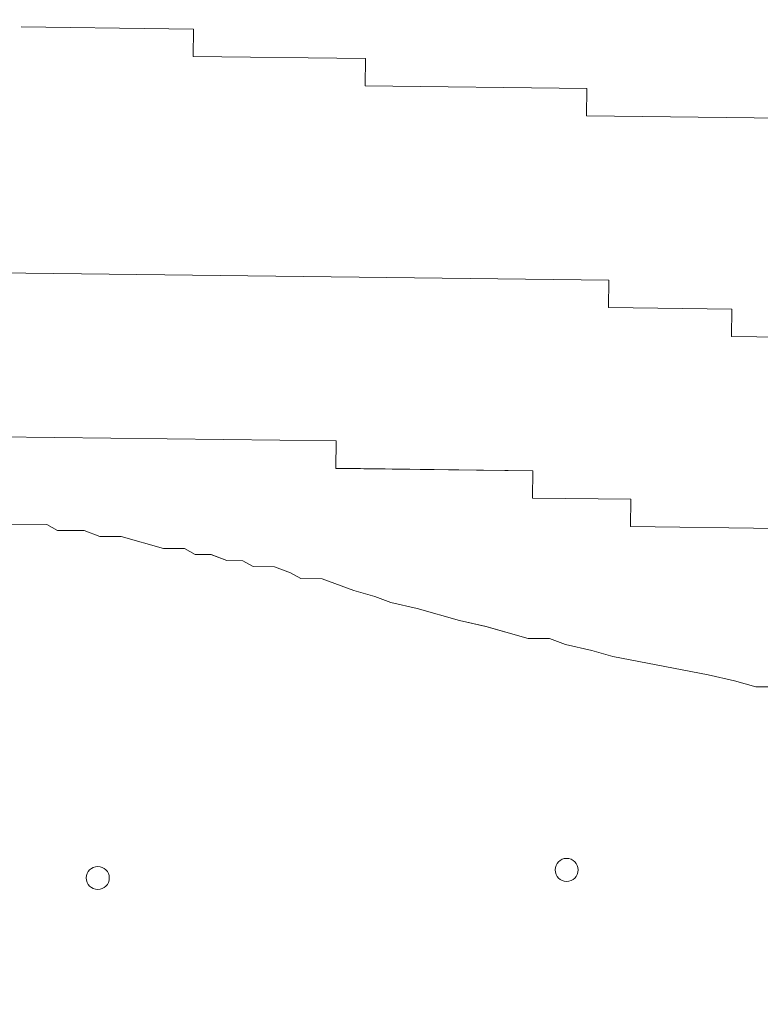
# Model space of a CAD drawing. Units: inches. Extents: x -466983 to 1020, y 324 to 318697.
# Tile 76 of 97: x 652.495 to 656.235, y 939.297 to 944.271. Entities that reach past the tile are written whole.
import ezdxf

# ---------------------------------------------------------------- set-up
doc = ezdxf.new("R2010")
doc.units = ezdxf.units.IN
doc.header["$MEASUREMENT"] = 0
doc.layers.add('A-FLOR-PATT', color=252, linetype='Continuous', lineweight=13)
doc.layers.add('A-FURN', color=8, linetype='Continuous', lineweight=18)

# ---------------------------------------------------------------- blocks, each defined once
blk = doc.blocks.new('L Shaped Sofa')
at = {"ltscale": 2}
for p, q in [((2395.89, 747.0093), (2396.0851, 747.0084)), ((2396.0851, 747.0084), (2396.28, 746.9532)), ((2396.28, 746.9532), (2396.5236, 746.8979)), ((2396.5236, 746.8979), (2397.4009, 746.7311)), ((2397.4009, 746.7311), (2397.5958, 746.676)), ((2397.5958, 746.676), (2397.8394, 746.6206)), ((2397.8394, 746.6206), (2397.9855, 746.5657)), ((2397.9855, 746.5657), (2398.1807, 746.5648)), ((2398.1807, 746.5648), (2398.5704, 746.4545)), ((2398.5704, 746.4545), (2398.814, 746.3992)), ((2398.814, 746.3992), (2399.2037, 746.2889)), ((2399.2037, 746.2889), (2399.4473, 746.2335)), ((2399.4473, 746.2335), (2399.5934, 746.1786)), ((2399.5934, 746.1786), (2399.7883, 746.1235)), ((2399.7883, 746.1235), (2400.0804, 746.0137)), ((2400.0804, 746.0137), (2400.2755, 746.0128)), ((2400.2755, 746.0128), (2400.3728, 745.9581)), ((2400.3728, 745.9581), (2400.5188, 745.9032)), ((2400.5188, 745.9032), (2400.714, 745.9023)), ((2400.714, 745.9023), (2400.8113, 745.8476)), ((2400.8113, 745.8476), (2400.9577, 745.8469)), ((2400.9577, 745.8469), (2401.1037, 745.792)), ((2401.1037, 745.792), (2401.2501, 745.7913)), ((2401.2501, 745.7913), (2401.3474, 745.7367)), ((2401.3474, 745.7367), (2401.5426, 745.7357)), ((2401.5426, 745.7357), (2401.9322, 745.6255)), ((2401.9322, 745.6255), (2402.1274, 745.6246)), ((2402.1274, 745.6246), (2402.2735, 745.5697)), ((2402.2735, 745.5697), (2402.5175, 745.5685)), ((2402.5175, 745.5685), (2402.6147, 745.5138)), ((2395.8772, 745.5504), (2397.2382, 745.5337)), ((2397.2382, 745.5337), (2397.2352, 745.2818)), ((2402.6147, 745.5138), (2403.0051, 745.512)), ((2397.2352, 745.2818), (2398.1425, 745.2707)), ((2398.1425, 745.2707), (2398.1394, 745.0188)), ((2398.1394, 745.0188), (2399.9541, 744.9967)), ((2399.9541, 744.9967), (2399.951, 744.7447)), ((2399.951, 744.7447), (2403.5804, 744.7004)), ((2395.1752, 743.7953), (2396.3094, 743.7814)), ((2396.3094, 743.7814), (2396.3063, 743.5295)), ((2396.3063, 743.5295), (2397.4405, 743.5157)), ((2397.4405, 743.5157), (2397.4374, 743.2638)), ((2397.4374, 743.2638), (2403.562, 743.1889)), ((2392.4285, 741.8133), (2397.6457, 741.7495)), ((2397.6457, 741.7495), (2397.6427, 741.4976)), ((2397.6427, 741.4976), (2399.6842, 741.4727)), ((2399.6842, 741.4727), (2399.6811, 741.2207)), ((2399.6811, 741.2207), (2401.269, 741.2013)), ((2401.269, 741.2013), (2401.2659, 740.9494)), ((2401.2659, 740.9494), (2401.7196, 740.9439)), ((2401.4927, 740.9467), (2402.8538, 740.93)), ((2401.7196, 740.9439), (2401.4927, 740.9467))]:
    blk.add_line(p, q, dxfattribs=at)
for centre, start, end in [((2402.1467, 748.7712), 90, 270), ((2402.1467, 748.7712), 270, 90), ((2397.8273, 748.697), 90, 270), ((2397.8273, 748.697), 270, 90)]:
    blk.add_arc(centre, 0.1062, start, end, dxfattribs=at)

msp = doc.modelspace()

# ---------------------------------------------------------------- hatches: boundary and pattern name
at = {"layer": 'A-FLOR-PATT', "transparency": 33554572}
h = msp.add_hatch(dxfattribs=at)
h.set_pattern_fill('ANSI37', color=256, scale=30)
h.set_pattern_definition([(45, (-1212.4137, -290.035), (-2.6516504, 2.6516504), []), (135, (-1212.4137, -290.035), (-2.6516504, -2.6516504), [])])
h.paths.add_polyline_path([(901.8057, 1075.9377), (900.6144, 1075.9377), (900.6144, 1065.3856), (899.391, 1065.3856), (898.0911, 1065.3856), (892.8356, 1058.7098, -0.258377), (892.1875, 1058.3509), (879.9848, 1058.3509, -0.20177), (879.4382, 1058.5808), (874.0812, 1065.3856), (872.7813, 1065.3856), (871.5579, 1065.3856), (871.5579, 1075.9377), (813.8057, 1075.9377), (813.8057, 1044.7922), (832.3947, 1044.7922, -0.394795), (848.6602, 1028.5356), (848.6602, 1009.9377), (901.8057, 1009.9377), (901.8057, 1015.9377), (901.3057, 1015.9377), (871.3057, 1015.9377), (871.3057, 1017.2502), (871.3344, 1017.2502, -0.401453), (901.3057, 1045.9377), (901.8057, 1045.9377)])
edge = h.paths.add_edge_path(flags=16)
edge.add_line((847.7731, 1068.9486), (847.7731, 1073.7088))
edge.add_arc((849.2269, 1073.7088), 1.4538, 90, 180, ccw=False)
edge.add_line((849.2269, 1075.1627), (864.4921, 1075.1627))
edge.add_arc((864.4921, 1073.7088), 1.4538, 0, 90, ccw=False)
edge.add_line((865.9459, 1073.7088), (865.9459, 1069.0035))
edge.add_arc((832.6447, 1068.9761), 33.3012, -20.61234, 0.04725, ccw=False)
edge.add_ellipse((856.8595, 1058.48), major_axis=(0, 10.2131), ratio=0.6859192, start_angle=100.00884, end_angle=259.99116, ccw=False)
edge.add_arc((881.0742, 1068.9761), 33.3012, 180.04725, 200.61234, ccw=False)
h.paths.add_polyline_path([(853.1456, 1066.4815), (853.1456, 1066.4534), (853.1463, 1066.4534, 0.433107), (852.9166, 1066.6849), (852.9166, 1066.4534), (853.1456, 1066.4534), (853.1456, 1066.4815), (853.088, 1066.6122, 0.697939), (852.6995, 1066.4534), (852.7003, 1066.4534), (852.7003, 1066.4815), (852.9166, 1067.0012), (852.9166, 1066.6849, -0.396254)], flags=0)
h.paths.add_polyline_path([(861.0187, 1066.4815), (861.0187, 1066.4534), (861.0194, 1066.4534, 0.416404), (860.8024, 1066.6849), (860.8024, 1066.4534), (861.0187, 1066.4534), (861.0187, 1066.4815), (860.9672, 1066.6053, 0.713344), (860.5726, 1066.4534), (860.5734, 1066.4534), (860.5734, 1066.4815), (860.8024, 1067.0012), (860.8024, 1066.6849, -0.379973)], flags=0)
edge = h.paths.add_edge_path(flags=0)
edge.add_spline(control_points=[(861.1298, 1065.7855), (861.4661, 1065.2478), (861.6134, 1065.0161), (861.9833, 1064.3736), (862.1924, 1063.9443), (862.5614, 1063.0391), (862.7212, 1062.5633), (862.9865, 1061.5781), (863.092, 1061.0689), (863.2452, 1060.031), (863.293, 1059.5025), (863.3295, 1058.4409), (863.3181, 1057.9078), (863.2366, 1056.8518), (863.1664, 1056.3289), (862.9695, 1055.308), (862.8427, 1054.8099), (862.5365, 1053.8522), (862.3571, 1053.3927), (861.9514, 1052.5249), (861.7251, 1052.1166), (861.233, 1051.3622), (860.9672, 1051.0162), (860.4048, 1050.3949), (860.1082, 1050.1197), (859.4937, 1049.6461), (859.1758, 1049.4476), (858.5276, 1049.1299), (858.1973, 1049.0107), (857.5315, 1048.8518), (857.1959, 1048.8121), (856.5249, 1048.812), (856.1894, 1048.8515), (855.5236, 1049.0101), (855.1933, 1049.1291), (854.545, 1049.4465), (854.2271, 1049.6449), (853.6124, 1050.1183), (853.3158, 1050.3933), (852.7533, 1051.0143), (852.4874, 1051.3602), (851.9952, 1052.1144), (851.7688, 1052.5225), (851.3629, 1053.3902), (851.1834, 1053.8496), (850.877, 1054.8071), (850.7501, 1055.3051), (850.553, 1056.326), (850.4827, 1056.8488), (850.401, 1057.9048), (850.3895, 1058.4379), (850.4257, 1059.4995), (850.4734, 1060.0281), (850.6265, 1061.066), (850.7318, 1061.5753), (850.9969, 1062.5605), (851.1567, 1063.0365), (851.5254, 1063.9418), (851.7345, 1064.3712), (852.1056, 1065.0164), (852.2544, 1065.2503), (852.6082, 1065.7335)], knot_values=[3.915332, 3.915332, 3.915332, 3.915332, 4.013468, 4.013468, 4.175532, 4.175532, 4.337596, 4.337596, 4.49966, 4.49966, 4.661724, 4.661724, 4.823788, 4.823788, 4.985852, 4.985852, 5.147916, 5.147916, 5.30998, 5.30998, 5.472044, 5.472044, 5.634109, 5.634109, 5.796173, 5.796173, 5.958237, 5.958237, 6.120301, 6.120301, 6.282365, 6.282365, 6.444429, 6.444429, 6.606493, 6.606493, 6.768557, 6.768557, 6.930621, 6.930621, 7.092685, 7.092685, 7.254749, 7.254749, 7.416813, 7.416813, 7.578878, 7.578878, 7.740942, 7.740942, 7.903006, 7.903006, 8.06507, 8.06507, 8.227134, 8.227134, 8.389198, 8.389198, 8.551262, 8.551262, 8.65037, 8.65037, 8.65037, 8.65037], degree=3, periodic=0)
edge.add_line((852.6421, 1065.7855), (861.1298, 1065.7855))
edge = h.paths.add_edge_path(flags=0)
edge.add_ellipse((856.8496, 1057.7432), major_axis=(0, 7.7921), ratio=0.687861, start_angle=0, end_angle=360)
h.paths.add_polyline_path([(848.8634, 1069.3891), (848.8634, 1073.9605, -0.414214), (849.9538, 1075.0508), (863.7652, 1075.0508, -0.414214), (864.8555, 1073.9605), (864.8555, 1069.3891, -0.388936), (864.5237, 1069.027, -0.043561), (849.1953, 1069.027, -0.388936)], flags=0)
h.paths.add_polyline_path([(853.1006, 1068.1122, -1), (852.6775, 1068.1122, -1)], flags=0)
edge = h.paths.add_edge_path(flags=0)
edge.add_ellipse((856.8595, 1057.3378), major_axis=(0, 2.207), ratio=0.657164, start_angle=0, end_angle=360)
h.paths.add_polyline_path([(861.0415, 1068.1122, -1), (860.6184, 1068.1122, -1)], flags=0)
edge = h.paths.add_edge_path()
edge.add_line((573.9537, 1057.3412), (573.9537, 1075.9377))
edge.add_line((573.9537, 1075.9377), (558.7308, 1075.9377))
edge.add_line((558.7308, 1075.9377), (558.7308, 1065.3856))
edge.add_line((558.7308, 1065.3856), (557.5074, 1065.3856))
edge.add_line((557.5074, 1065.3856), (556.2075, 1065.3856))
edge.add_line((556.2075, 1065.3856), (550.952, 1058.7098))
edge.add_arc((550.3039, 1059.1155), 0.7646, 270, 327.9483, ccw=False)
edge.add_line((550.3039, 1058.3509), (538.1012, 1058.3509))
edge.add_arc((538.1012, 1059.1155), 0.7646, 224.3704, 270, ccw=False)
edge.add_line((537.5546, 1058.5808), (532.1976, 1065.3856))
edge.add_line((532.1976, 1065.3856), (530.8977, 1065.3856))
edge.add_line((530.8977, 1065.3856), (529.6743, 1065.3856))
edge.add_line((529.6743, 1065.3856), (529.6743, 1075.9377))
edge.add_line((529.6743, 1075.9377), (520.8057, 1075.9377))
edge.add_line((520.8057, 1075.9377), (520.8057, 1045.9377))
edge.add_line((520.8057, 1045.9377), (521.3057, 1045.9377))
edge.add_arc((521.3057, 1015.9377), 30, 2.50749, 90, ccw=False)
edge.add_line((551.277, 1017.2502), (551.3057, 1017.2502))
edge.add_line((551.3057, 1017.2502), (551.3057, 1015.9377))
edge.add_line((551.3057, 1015.9377), (520.8057, 1015.9377))
edge.add_line((520.8057, 1015.9377), (520.8057, 1009.9377))
edge.add_line((520.8057, 1009.9377), (559.1913, 1010.4022))
edge.add_arc((559.1913, 1011.856), 1.4538, 180, 270, ccw=False)
edge.add_line((557.7375, 1011.856), (557.7375, 1016.5613))
edge.add_arc((591.0386, 1016.5888), 33.3012, 159.38766, 180.04725, ccw=False)
edge.add_ellipse((566.8239, 1027.0848), major_axis=(0, 10.2131), ratio=0.6859192, start_angle=280.00884, end_angle=439.99116, ccw=False)
edge.add_arc((542.6091, 1016.5888), 33.3012, 0.04725, 20.61234, ccw=False)
edge.add_line((575.9103, 1016.6162), (575.9103, 1011.856))
edge.add_arc((574.4565, 1011.856), 1.4538, -90, 0, ccw=False)
edge.add_line((574.4565, 1010.4022), (608.8057, 1009.9377))
edge.add_line((608.8057, 1009.9377), (608.8057, 1041.0857))
edge.add_line((608.8057, 1041.0857), (590.2179, 1041.0857))
edge.add_arc((590.775, 1057.9074), 16.8309, 181.92775, 268.10321, ccw=False)
edge = h.paths.add_edge_path()
edge.add_ellipse((494.2443, 583.6204), major_axis=(0, 10.2131), ratio=0.6859192, start_angle=280.00884, end_angle=439.99116, ccw=False)
edge.add_arc((470.0296, 573.1243), 33.3012, 0.04725, 20.61234, ccw=False)
edge.add_line((503.3307, 573.1518), (503.3307, 568.3916))
edge.add_arc((501.8769, 568.3916), 1.4538, -90, 0, ccw=False)
edge.add_line((501.8769, 566.9377), (539.8057, 566.9377))
edge.add_line((539.8057, 566.9377), (539.8057, 572.9377))
edge.add_line((539.8057, 572.9377), (539.3057, 572.9377))
edge.add_line((539.3057, 572.9377), (509.3057, 572.9377))
edge.add_line((509.3057, 572.9377), (509.3057, 574.2502))
edge.add_line((509.3057, 574.2502), (509.3344, 574.2502))
edge.add_arc((539.3057, 572.9377), 30, 90, 177.49251, ccw=False)
edge.add_line((539.3057, 602.9377), (539.8057, 602.9377))
edge.add_line((539.8057, 602.9377), (539.8057, 626.9377))
edge.add_line((539.8057, 626.9377), (531.7718, 626.9377))
edge.add_line((531.7718, 626.9377), (531.7718, 616.3856))
edge.add_line((531.7718, 616.3856), (530.5484, 616.3856))
edge.add_line((530.5484, 616.3856), (529.2485, 616.3856))
edge.add_line((529.2485, 616.3856), (523.7105, 609.3509))
edge.add_line((523.7105, 609.3509), (510.7766, 609.3509))
edge.add_line((510.7766, 609.3509), (505.2386, 616.3856))
edge.add_line((505.2386, 616.3856), (503.9387, 616.3856))
edge.add_line((503.9387, 616.3856), (502.7153, 616.3856))
edge.add_line((502.7153, 616.3856), (502.7153, 626.9377))
edge.add_line((502.7153, 626.9377), (481.6983, 626.9377))
edge.add_line((481.6983, 626.9377), (481.6983, 610.995))
edge.add_arc((467.2703, 611.4728), 14.4359, 271.92775, 358.10321, ccw=False)
edge.add_line((467.7559, 597.0451), (451.8057, 597.0451))
edge.add_line((451.8057, 597.0451), (451.8057, 584.4035))
edge.add_line((451.8057, 584.4035), (451.8057, 566.9377))
edge.add_line((451.8057, 566.9377), (486.6117, 566.9377))
edge.add_arc((486.6117, 568.3916), 1.4538, 180, 270, ccw=False)
edge.add_line((485.1579, 568.3916), (485.1579, 573.0969))
edge.add_arc((518.4591, 573.1243), 33.3012, 159.38766, 180.04725, ccw=False)
h.paths.add_polyline_path([(836.2609, 1020.7328), (879.8898, 1020.7328), (879.8898, 1039.3902), (836.2609, 1039.3902)], flags=25)
h.paths.add_polyline_path([(549.9851, 1036.7492), (593.614, 1036.7492), (593.614, 1055.4065), (549.9851, 1055.4065)], flags=24)
h.paths.add_polyline_path([(475.123, 595.5959), (518.752, 595.5959), (518.752, 614.2532), (475.123, 614.2532)], flags=24)
h = msp.add_hatch(dxfattribs=at)
h.set_pattern_fill('ANSI37', color=256, scale=20)
h.set_pattern_definition([(45, (-1212.4137, -290.035), (-1.767767, 1.767767), []), (135, (-1212.4137, -290.035), (-1.767767, -1.767767), [])])
h.paths.add_polyline_path([(809.8057, 870.9377), (809.8057, 888.1519), (806.9985, 888.1519), (802.6624, 888.1519), (789.3832, 888.1519), (786.2846, 888.1519, -0.414214), (785.4991, 888.9374), (785.4991, 900.1959), (785.4991, 908.4696, -0.414214), (786.8082, 909.7787, -0.414214), (785.4991, 911.0878), (785.4991, 929.1015, -0.414214), (786.8082, 930.4106, -0.414214), (785.4991, 931.7197), (785.4991, 931.9039, -0.414214), (784.19, 930.5948), (766.7223, 930.5948, -0.412359), (765.4132, 931.8956, -0.413741), (764.1145, 930.5782), (744.5781, 930.422, -0.416556), (743.7864, 931.2075), (743.7864, 933.5153), (742.2154, 933.5153), (742.2154, 952.024, -0.001344), (743.7864, 952.1998), (743.7864, 953.9377), (678.5915, 953.9377), (678.5915, 951.1305), (678.5915, 946.7945), (678.5915, 933.5153), (678.5915, 930.4166, -0.414214), (677.806, 929.6312), (666.5475, 929.6312), (658.2738, 929.6312, -0.414214), (656.9647, 930.9403, -0.414214), (655.6556, 929.6312), (637.6419, 929.6312, -0.414214), (636.3328, 930.9403, -0.414214), (635.0237, 929.6312), (634.8395, 929.6312, -0.414214), (636.1486, 928.322), (636.1486, 910.8544, -0.412359), (634.8478, 909.5452, -0.413741), (636.1653, 908.2466), (636.3214, 888.7102, -0.416556), (635.5359, 887.9184), (633.2281, 887.9184), (633.2281, 886.3475), (614.7194, 886.3475, -0.001344), (614.5436, 887.9184), (612.8057, 887.9184), (612.8057, 834.9377), (612.8057, 752.9377), (612.8057, 748.9377), (612.8057, 697.9377), (654.8057, 697.9377), (654.8057, 701.9377), (715.8057, 701.9377), (715.8057, 737.4353), (774.2918, 737.4353), (774.2918, 795.9377), (809.8057, 795.9377)])
h.paths.add_polyline_path([(679.2761, 849.5757, 0.102523), (682.1475, 849.2608, -0.080461), (694.5428, 849.7725, -0.283899), (694.4822, 849.0082, 0.136605), (694.4068, 848.8103, -0.030441), (694.5428, 846.8929), (694.5428, 842.6198), (694.5428, 838.3466, -0.028219), (694.4246, 836.5684), (694.425, 836.5684, 0.196187), (694.4456, 836.2708, -0.302897), (694.5428, 835.467, -0.080461), (682.1475, 835.9787, 0.102523), (679.2761, 835.6638, -0.58611), (678.6457, 836.0169), (678.6457, 849.2227, -0.58611)], flags=16)
h.paths.add_polyline_path([(679.5173, 848.6515, 0.699597), (679.476, 848.6342, 1.20716), (679.1935, 848.7422, 0.010621)], flags=0)
h.paths.add_polyline_path([(679.4923, 836.5608, -0.013798), (679.9178, 836.6594, -0.071703), (682.8533, 837.1434, -0.165743), (682.1665, 839.1006), (682.1665, 842.6094), (682.1665, 846.0603, -0.240616), (683.4733, 848.6767, -0.068263), (693.9295, 849.0082), (693.7875, 848.7083), (693.7875, 849.0228, 0.067332), (683.4733, 848.6767, 0.240616), (682.1665, 846.0603), (682.1665, 842.6094), (682.1665, 839.1006, 0.23459), (683.461, 836.5513, 0.068093), (693.7875, 836.1955), (693.7875, 836.5104), (693.9296, 836.2102, -0.077215), (682.2421, 836.7815, 0.086627), (679.5283, 836.5701, -0.628402), (679.5029, 836.5735), (679.5029, 836.6071, 0.910458)], flags=0)
h.paths.add_polyline_path([(679.476, 848.6364), (679.2069, 848.647), (679.2069, 836.5718, 0.913566), (679.3645, 836.5861), (679.476, 836.5824)], flags=0)
h.paths.add_polyline_path([(679.2761, 829.8604, 0.102523), (682.1475, 829.5455, -0.080461), (694.5428, 830.0572, -0.283899), (694.4822, 829.2929, 0.136605), (694.4068, 829.095, -0.030441), (694.5428, 827.1776), (694.5428, 822.9045), (694.5428, 818.6314, -0.028219), (694.4246, 816.8531), (694.425, 816.8532, 0.196187), (694.4456, 816.5555, -0.302897), (694.5428, 815.7517, -0.080461), (682.1475, 816.2635, 0.102523), (679.2761, 815.9485, -0.58611), (678.6457, 816.3016), (678.6457, 829.5074, -0.58611)], flags=16)
h.paths.add_polyline_path([(679.5173, 828.9362, 0.699597), (679.476, 828.9189, 1.20716), (679.1935, 829.0269, 0.010621)], flags=0)
h.paths.add_polyline_path([(679.4923, 816.8456, -0.013798), (679.9178, 816.9441, -0.071703), (682.8533, 817.4281, -0.165743), (682.1665, 819.3853), (682.1665, 822.8941), (682.1665, 826.345, -0.240616), (683.4733, 828.9614, -0.068263), (693.9295, 829.2929), (693.7875, 828.9931), (693.7875, 829.3076, 0.067332), (683.4733, 828.9614, 0.240616), (682.1665, 826.345), (682.1665, 822.8941), (682.1665, 819.3853, 0.23459), (683.461, 816.836, 0.068093), (693.7875, 816.4802), (693.7875, 816.7952), (693.9296, 816.4949, -0.077215), (682.2421, 817.0662, 0.086627), (679.5283, 816.8549, -0.628402), (679.5029, 816.8582), (679.5029, 816.8918, 0.910458)], flags=0)
h.paths.add_polyline_path([(679.476, 828.9211), (679.2069, 828.9317), (679.2069, 816.8565, 0.913566), (679.3645, 816.8708), (679.476, 816.8671)], flags=0)
h.paths.add_polyline_path([(679.2761, 810.1451, 0.102523), (682.1475, 809.8302, -0.080461), (694.5428, 810.342, -0.3023), (694.4466, 809.5394, 0.10023), (694.4058, 809.3878, -0.03057), (694.5428, 807.4623), (694.5428, 803.1892), (694.5428, 798.9161, -0.03057), (694.4058, 796.9906, 0.10023), (694.4466, 796.839, -0.3023), (694.5428, 796.0365, -0.080461), (682.1475, 796.5482, 0.102523), (679.2761, 796.2333, -0.58611), (678.6457, 796.5863), (678.6457, 809.7921, -0.58611)], flags=16)
h.paths.add_polyline_path([(679.5173, 809.2417, 0.699597), (679.476, 809.2244, 1.20716), (679.1935, 809.3324, 0.010621)], flags=0)
h.paths.add_polyline_path([(679.4923, 797.151, -0.013798), (679.9178, 797.2496, -0.071703), (682.8533, 797.7336, -0.165743), (682.1665, 799.6908), (682.1665, 803.1996), (682.1665, 806.6505, -0.239349), (683.461, 809.2577, -0.072465), (694.4468, 809.5405, 0.197932), (694.425, 809.2405), (693.7875, 809.2985), (693.7875, 809.6135, 0.068093), (683.461, 809.2577, 0.239349), (682.1665, 806.6505), (682.1665, 803.1996), (682.1665, 799.6908, 0.235854), (683.4733, 797.1323, 0.067332), (693.7875, 796.7861), (693.7875, 797.1006), (694.425, 797.1586, 0.197932), (694.4468, 796.8586, -0.080419), (682.1557, 797.3795, 0.083867), (679.5283, 797.1603, -0.628402), (679.5029, 797.1637), (679.5029, 797.1973, 0.910458)], flags=0)
h.paths.add_polyline_path([(679.2069, 809.2372), (679.2069, 797.162, 0.913566), (679.3645, 797.1763), (679.476, 797.1726), (679.476, 809.2266)], flags=0)
h.paths.add_polyline_path([(695.3643, 853.2989), (728.2231, 853.2989), (728.2231, 771.1519), (695.3643, 771.1519)], flags=16)
h.paths.add_polyline_path([(696.0215, 852.6417), (727.5659, 852.6417), (727.5659, 771.809), (696.0215, 771.809)], flags=0)
h.paths.add_polyline_path([(679.2761, 788.7869, 0.102523), (682.1475, 788.472, -0.080461), (694.5428, 788.9837, -0.3023), (694.4466, 788.1812, 0.10023), (694.4058, 788.0296, -0.03057), (694.5428, 786.1041), (694.5428, 781.831), (694.5428, 777.5578, -0.03057), (694.4058, 775.6323, 0.10023), (694.4466, 775.4808, -0.3023), (694.5428, 774.6782, -0.080461), (682.1475, 775.19, 0.102523), (679.2761, 774.875, -0.58611), (678.6457, 775.2281), (678.6457, 788.4339, -0.58611)], flags=16)
h.paths.add_polyline_path([(679.5173, 787.8834, 0.699597), (679.476, 787.8662, 1.20716), (679.1935, 787.9742, 0.010621)], flags=0)
h.paths.add_polyline_path([(679.4923, 775.7928, -0.013798), (679.9178, 775.8914, -0.071703), (682.8533, 776.3753, -0.165743), (682.1665, 778.3325), (682.1665, 781.8414), (682.1665, 785.2922, -0.239349), (683.461, 787.8995, -0.072465), (694.4468, 788.1823, 0.197932), (694.425, 787.8823), (693.7875, 787.9403), (693.7875, 788.2553, 0.068093), (683.461, 787.8995, 0.239349), (682.1665, 785.2922), (682.1665, 781.8414), (682.1665, 778.3325, 0.235854), (683.4733, 775.7741, 0.067332), (693.7875, 775.4279), (693.7875, 775.7424), (694.425, 775.8004, 0.197932), (694.4468, 775.5004, -0.080419), (682.1557, 776.0212, 0.083867), (679.5283, 775.8021, -0.628402), (679.5029, 775.8054), (679.5029, 775.8391, 0.910458)], flags=0)
h.paths.add_polyline_path([(679.2069, 787.8789), (679.2069, 775.8038, 0.913566), (679.3645, 775.818), (679.476, 775.8144), (679.476, 787.8684)], flags=0)
h.paths.add_polyline_path([(704.641, 854.1204, -0.080461), (705.1527, 866.5157, 0.102523), (704.8378, 869.3871, -0.58611), (705.1908, 870.0174), (718.3966, 870.0174, -0.58611), (718.7496, 869.3871, 0.102523), (718.4347, 866.5157, -0.080461), (718.9465, 854.1204, -0.3023), (718.1439, 854.2166, 0.10023), (717.9924, 854.2574, -0.03057), (716.0668, 854.1204), (711.7937, 854.1204), (707.5206, 854.1204, -0.03057), (705.5951, 854.2574, 0.10023), (705.4435, 854.2166, -0.3023)], flags=16)
h.paths.add_polyline_path([(717.8462, 869.1459, 0.699597), (717.8289, 869.1872, 1.20716), (717.9369, 869.4697, 0.010621)], flags=0)
h.paths.add_polyline_path([(705.4631, 854.2164, -0.080419), (705.984, 866.5074, 0.083867), (705.7648, 869.1349, -0.628402), (705.7682, 869.1603), (705.8018, 869.1603, 0.910458), (705.7555, 869.1709, -0.013798), (705.8541, 868.7454, -0.071703), (706.3381, 865.8099, -0.165743), (708.2953, 866.4967), (711.8041, 866.4967), (715.255, 866.4967, -0.239349), (717.8622, 865.2022, -0.072465), (718.145, 854.2164, 0.197932), (717.845, 854.2382), (717.903, 854.8757), (718.218, 854.8757, 0.068093), (717.8622, 865.2022, 0.239349), (715.255, 866.4967), (711.8041, 866.4967), (708.2953, 866.4967, 0.235854), (705.7368, 865.1898, 0.067332), (705.3906, 854.8757), (705.7051, 854.8757), (705.7631, 854.2382, 0.197932)], flags=16)
h.paths.add_polyline_path([(705.7665, 869.4563, 0.913566), (705.7808, 869.2987), (705.7771, 869.1872), (717.8311, 869.1872), (717.8417, 869.4563)], flags=0)
h.paths.add_polyline_path([(729.0446, 842.6198), (729.0446, 846.8929, -0.03057), (729.1817, 848.8184, 0.10023), (729.1408, 848.9699, -0.3023), (729.0446, 849.7725, -0.080461), (741.4399, 849.2608, 0.102523), (744.3113, 849.5757, -0.58611), (744.9417, 849.2227), (744.9417, 836.0169, -0.58611), (744.3113, 835.6638, 0.102523), (741.4399, 835.9787, -0.080461), (729.0446, 835.467, -0.3023), (729.1408, 836.2696, 0.10023), (729.1817, 836.4211, -0.03057), (729.0446, 838.3466)], flags=16)
h.paths.add_polyline_path([(744.1115, 836.5846, 1.20716), (744.3939, 836.4766, 0.010621), (744.0701, 836.5673, 0.699597)], flags=0)
h.paths.add_polyline_path([(729.1407, 836.2684, 0.197932), (729.1624, 836.5684), (729.7999, 836.5104), (729.7999, 836.1955, 0.068093), (740.1264, 836.5513, 0.239349), (741.4209, 839.1585), (741.4209, 842.6094), (741.4209, 846.1182, 0.235854), (740.1141, 848.6767, 0.067332), (729.7999, 849.0228), (729.7999, 848.7083), (729.1624, 848.6503, 0.197932), (729.1407, 848.9504, -0.080419), (741.4317, 848.4295, 0.083867), (744.0591, 848.6486, -0.628402), (744.0845, 848.6453), (744.0845, 848.6117, 0.910458), (744.0951, 848.6579, -0.013798), (743.6696, 848.5594, -0.071703), (740.7341, 848.0754, -0.165743), (741.4209, 846.1182), (741.4209, 842.6094), (741.4209, 839.1585, -0.239349), (740.1264, 836.5513, -0.072465)], flags=0)
h.paths.add_polyline_path([(729.0446, 830.0572, -0.080461), (741.4399, 829.5455, 0.102523), (744.3113, 829.8604, -0.58611), (744.9417, 829.5074), (744.9417, 816.3016, -0.58611), (744.3113, 815.9485, 0.102523), (741.4399, 816.2635, -0.080461), (729.0446, 815.7517, -0.3023), (729.1408, 816.5543, 0.10023), (729.1817, 816.7058, -0.03057), (729.0446, 818.6314), (729.0446, 822.9045), (729.0446, 827.1776, -0.03057), (729.1817, 829.1031, 0.10023), (729.1408, 829.2547, -0.3023)], flags=16)
h.paths.add_polyline_path([(744.1115, 816.8693, 1.20716), (744.3939, 816.7613, 0.010621), (744.0701, 816.852, 0.699597)], flags=0)
h.paths.add_polyline_path([(729.1407, 829.2351, -0.080419), (741.4317, 828.7142, 0.083867), (744.0591, 828.9334, -0.628402), (744.0845, 828.93), (744.0845, 828.8964, 0.910458), (744.0951, 828.9427, -0.013798), (743.6696, 828.8441, -0.071703), (740.7341, 828.3601, -0.165743), (741.4209, 826.4029), (741.4209, 822.8941), (741.4209, 819.4432, -0.239349), (740.1264, 816.836, -0.072465), (729.1407, 816.5531, 0.197932), (729.1624, 816.8532), (729.7999, 816.7952), (729.7999, 816.4802, 0.068093), (740.1264, 816.836, 0.239349), (741.4209, 819.4432), (741.4209, 822.8941), (741.4209, 826.4029, 0.235854), (740.1141, 828.9614, 0.067332), (729.7999, 829.3076), (729.7999, 828.9931), (729.1624, 828.9351, 0.197932)], flags=16)
h.paths.add_polyline_path([(729.0446, 810.342, -0.080461), (741.4399, 809.8302, 0.102523), (744.3113, 810.1451, -0.58611), (744.9417, 809.7921), (744.9417, 796.5863, -0.58611), (744.3113, 796.2333, 0.102523), (741.4399, 796.5482, -0.080461), (729.0446, 796.0365, -0.283899), (729.1052, 796.8007, 0.136605), (729.1806, 796.9987, -0.030441), (729.0446, 798.9161), (729.0446, 803.1892), (729.0446, 807.4623, -0.028219), (729.1628, 809.2406), (729.1624, 809.2405, 0.196187), (729.1418, 809.5382, -0.302897)], flags=16)
h.paths.add_polyline_path([(744.1115, 797.1748, 1.20716), (744.3939, 797.0668, 0.010621), (744.0701, 797.1575, 0.699597)], flags=0)
h.paths.add_polyline_path([(741.3453, 809.0275, 0.086627), (744.0591, 809.2388, -0.628402), (744.0845, 809.2355), (744.0845, 809.2019, 0.910458), (744.0951, 809.2481, -0.013798), (743.6696, 809.1496, -0.071703), (740.7341, 808.6656, -0.165743), (741.4209, 806.7084), (741.4209, 803.1996), (741.4209, 799.7487, -0.240616), (740.1141, 797.1323, -0.068263), (729.658, 796.8008), (729.7999, 797.1006), (729.7999, 796.7861, 0.067332), (740.1141, 797.1323, 0.240616), (741.4209, 799.7487), (741.4209, 803.1996), (741.4209, 806.7084, 0.23459), (740.1264, 809.2577, 0.068093), (729.7999, 809.6135), (729.7999, 809.2985), (729.6578, 809.5988, -0.077215)], flags=0)
h.paths.add_polyline_path([(704.641, 770.3304, -0.283899), (705.4053, 770.2697, 0.136605), (705.6032, 770.1944, -0.030441), (707.5206, 770.3304), (711.7937, 770.3304), (716.0668, 770.3304, -0.028219), (717.8451, 770.2122), (717.845, 770.2126, 0.196187), (718.1427, 770.2331, -0.302897), (718.9465, 770.3304, -0.080461), (718.4347, 757.9351, 0.102523), (718.7496, 755.0637, -0.58611), (718.3966, 754.4333), (705.1908, 754.4333, -0.58611), (704.8378, 755.0637, 0.102523), (705.1527, 757.9351, -0.080461)], flags=16)
h.paths.add_polyline_path([(705.762, 755.3048, 0.699597), (705.7793, 755.2635, 1.20716), (705.6713, 754.9811, 0.010621)], flags=0)
h.paths.add_polyline_path([(705.4053, 769.717), (705.7051, 769.5751), (705.3906, 769.5751, 0.067332), (705.7368, 759.2609, 0.240616), (708.3532, 757.954), (711.8041, 757.954), (715.3129, 757.954, 0.23459), (717.8622, 759.2485, 0.068093), (718.218, 769.5751), (717.903, 769.5751), (718.2033, 769.7172, -0.077215), (717.632, 758.0297, 0.086627), (717.8433, 755.3159, -0.628402), (717.84, 755.2904), (717.8064, 755.2904, 0.910458), (717.8526, 755.2799, -0.013798), (717.7541, 755.7053, -0.071703), (717.2701, 758.6409, -0.165743), (715.3129, 757.954), (711.8041, 757.954), (708.3532, 757.954, -0.240616), (705.7368, 759.2609, -0.068263)], flags=0)
h.paths.add_polyline_path([(729.0446, 788.9837, -0.080461), (741.4399, 788.472, 0.102523), (744.3113, 788.7869, -0.58611), (744.9417, 788.4339), (744.9417, 775.2281, -0.58611), (744.3113, 774.875, 0.102523), (741.4399, 775.19, -0.080461), (729.0446, 774.6782, -0.283899), (729.1052, 775.4425, 0.136605), (729.1806, 775.6405, -0.030441), (729.0446, 777.5578), (729.0446, 781.831), (729.0446, 786.1041, -0.028219), (729.1628, 787.8823), (729.1624, 787.8823, 0.196187), (729.1418, 788.1799, -0.302897)], flags=16)
h.paths.add_polyline_path([(744.1115, 775.8165, 1.20716), (744.3939, 775.7086, 0.010621), (744.0701, 775.7993, 0.699597)], flags=0)
h.paths.add_polyline_path([(741.3453, 787.6692, 0.086627), (744.0591, 787.8806, -0.628402), (744.0845, 787.8773), (744.0845, 787.8437, 0.910458), (744.0951, 787.8899, -0.013798), (743.6696, 787.7913, -0.071703), (740.7341, 787.3074, -0.165743), (741.4209, 785.3502), (741.4209, 781.8414), (741.4209, 778.3905, -0.240616), (740.1141, 775.7741, -0.068263), (729.658, 775.4425), (729.7999, 775.7424), (729.7999, 775.4279, 0.067332), (740.1141, 775.7741, 0.240616), (741.4209, 778.3905), (741.4209, 781.8414), (741.4209, 785.3502, 0.23459), (740.1264, 787.8995, 0.068093), (729.7999, 788.2553), (729.7999, 787.9403), (729.6578, 788.2405, -0.077215)], flags=0)
h.paths.add_polyline_path([(744.1115, 848.6364), (744.1115, 836.5824), (744.3805, 836.5718), (744.3805, 848.647, 0.913566), (744.2229, 848.6327)], flags=0)
h.paths.add_polyline_path([(744.2229, 828.9174), (744.1115, 828.9211), (744.1115, 816.8671), (744.3805, 816.8565), (744.3805, 828.9317, 0.913566)], flags=0)
h.paths.add_polyline_path([(717.8311, 755.2635), (705.7771, 755.2635), (705.7665, 754.9945), (717.8417, 754.9945, 0.913566), (717.8274, 755.1521)], flags=0)
h.paths.add_polyline_path([(744.2229, 809.2229), (744.1115, 809.2266), (744.1115, 797.1726), (744.3805, 797.162), (744.3805, 809.2372, 0.913566)], flags=0)
h.paths.add_polyline_path([(744.1115, 787.8684), (744.1115, 775.8144), (744.3805, 775.8038), (744.3805, 787.8789, 0.913566), (744.2229, 787.8647)], flags=0)
h.paths.add_polyline_path([(678.8774, 877.1228), (737.6127, 877.1228), (737.6127, 899.5116), (678.8774, 899.5116)], flags=24)

# ---------------------------------------------------------------- linework, layer by layer
at = {"layer": 'A-FURN', "ltscale": 2}
for p, q in [((653.2476, 944.2249), (652.5014, 944.234)), ((653.2476, 944.2249), (652.5014, 944.234)), ((653.2476, 944.2249), (652.5014, 944.234)), ((653.2476, 944.2249), (652.5014, 944.234)), ((653.2476, 944.2249), (652.5014, 944.234)), ((653.2476, 944.2249), (652.5014, 944.234)), ((653.1232, 944.2264), (653.2476, 944.2249)), ((653.3719, 944.2233), (653.1232, 944.2264)), ((653.1232, 944.2264), (653.2476, 944.2249)), ((653.3719, 944.2233), (653.1232, 944.2264)), ((653.1232, 944.2264), (653.2476, 944.2249)), ((653.3719, 944.2233), (653.1232, 944.2264)), ((653.1232, 944.2264), (653.2476, 944.2249)), ((653.3719, 944.2233), (653.1232, 944.2264)), ((653.1232, 944.2264), (653.2476, 944.2249)), ((653.3719, 944.2233), (653.1232, 944.2264)), ((653.1232, 944.2264), (653.2476, 944.2249)), ((653.3719, 944.2233), (653.1232, 944.2264)), ((653.3702, 944.0852), (653.3719, 944.2233)), ((653.3702, 944.0852), (653.3719, 944.2233)), ((653.3702, 944.0852), (653.3719, 944.2233)), ((653.3702, 944.0852), (653.3719, 944.2233)), ((653.3702, 944.0852), (653.3719, 944.2233)), ((653.3702, 944.0852), (653.3719, 944.2233)), ((654.2407, 944.0746), (653.3702, 944.0852)), ((654.2407, 944.0746), (653.3702, 944.0852)), ((654.2407, 944.0746), (653.3702, 944.0852)), ((654.2407, 944.0746), (653.3702, 944.0852)), ((654.2407, 944.0746), (653.3702, 944.0852)), ((654.2407, 944.0746), (653.3702, 944.0852)), ((654.239, 943.9365), (654.2407, 944.0746)), ((654.239, 943.9365), (654.2407, 944.0746)), ((654.239, 943.9365), (654.2407, 944.0746)), ((654.239, 943.9365), (654.2407, 944.0746)), ((654.239, 943.9365), (654.2407, 944.0746)), ((654.239, 943.9365), (654.2407, 944.0746)), ((655.3582, 943.9228), (654.239, 943.9365)), ((655.3582, 943.9228), (654.239, 943.9365)), ((655.3582, 943.9228), (654.239, 943.9365)), ((655.3582, 943.9228), (654.239, 943.9365)), ((655.3582, 943.9228), (654.239, 943.9365)), ((655.3582, 943.9228), (654.239, 943.9365)), ((655.3565, 943.7847), (655.3582, 943.9228)), ((655.3565, 943.7847), (655.3582, 943.9228)), ((655.3565, 943.7847), (655.3582, 943.9228)), ((655.3565, 943.7847), (655.3582, 943.9228)), ((655.3565, 943.7847), (655.3582, 943.9228)), ((655.3565, 943.7847), (655.3582, 943.9228)), ((658.2167, 943.7498), (655.3565, 943.7847)), ((658.2167, 943.7498), (655.3565, 943.7847)), ((658.2167, 943.7498), (655.3565, 943.7847)), ((658.2167, 943.7498), (655.3565, 943.7847)), ((658.2167, 943.7498), (655.3565, 943.7847)), ((658.2167, 943.7498), (655.3565, 943.7847)), ((655.4708, 942.9546), (652.1132, 942.9956)), ((655.4708, 942.9546), (652.1132, 942.9956)), ((655.4708, 942.9546), (652.1132, 942.9956)), ((655.4708, 942.9546), (652.1132, 942.9956)), ((655.4708, 942.9546), (652.1132, 942.9956)), ((655.4708, 942.9546), (652.1132, 942.9956)), ((655.4691, 942.8165), (655.4708, 942.9546)), ((655.4691, 942.8165), (655.4708, 942.9546)), ((655.4691, 942.8165), (655.4708, 942.9546)), ((655.4691, 942.8165), (655.4708, 942.9546)), ((655.4691, 942.8165), (655.4708, 942.9546)), ((655.4691, 942.8165), (655.4708, 942.9546)), ((656.0909, 942.8089), (655.4691, 942.8165)), ((656.0909, 942.8089), (655.4691, 942.8165)), ((656.0909, 942.8089), (655.4691, 942.8165)), ((656.0909, 942.8089), (655.4691, 942.8165)), ((656.0909, 942.8089), (655.4691, 942.8165)), ((656.0909, 942.8089), (655.4691, 942.8165)), ((656.0892, 942.6708), (656.0909, 942.8089)), ((656.0892, 942.6708), (656.0909, 942.8089)), ((656.0892, 942.6708), (656.0909, 942.8089)), ((656.0892, 942.6708), (656.0909, 942.8089)), ((656.0892, 942.6708), (656.0909, 942.8089)), ((656.0892, 942.6708), (656.0909, 942.8089)), ((656.711, 942.6632), (656.0892, 942.6708)), ((656.711, 942.6632), (656.0892, 942.6708)), ((656.711, 942.6632), (656.0892, 942.6708)), ((656.711, 942.6632), (656.0892, 942.6708)), ((656.711, 942.6632), (656.0892, 942.6708)), ((656.711, 942.6632), (656.0892, 942.6708)), ((654.0927, 942.1427), (652.1031, 942.167)), ((654.0927, 942.1427), (652.1031, 942.167)), ((654.0927, 942.1427), (652.1031, 942.167)), ((654.0927, 942.1427), (652.1031, 942.167)), ((654.0927, 942.1427), (652.1031, 942.167)), ((654.0927, 942.1427), (652.1031, 942.167)), ((654.0911, 942.0046), (654.0927, 942.1427)), ((654.0911, 942.0046), (654.0927, 942.1427)), ((654.0911, 942.0046), (654.0927, 942.1427)), ((654.0911, 942.0046), (654.0927, 942.1427)), ((654.0911, 942.0046), (654.0927, 942.1427)), ((654.0911, 942.0046), (654.0927, 942.1427)), ((655.0859, 941.9924), (654.0911, 942.0046)), ((655.0859, 941.9924), (654.0911, 942.0046)), ((655.0859, 941.9924), (654.0911, 942.0046)), ((655.0859, 941.9924), (654.0911, 942.0046)), ((655.0859, 941.9924), (654.0911, 942.0046)), ((655.0859, 941.9924), (654.0911, 942.0046)), ((655.0842, 941.8543), (655.0859, 941.9924)), ((655.0842, 941.8543), (655.0859, 941.9924)), ((655.0842, 941.8543), (655.0859, 941.9924)), ((655.0842, 941.8543), (655.0859, 941.9924)), ((655.0842, 941.8543), (655.0859, 941.9924)), ((655.0842, 941.8543), (655.0859, 941.9924)), ((655.5816, 941.8483), (655.0842, 941.8543)), ((655.5816, 941.8483), (655.0842, 941.8543)), ((655.5816, 941.8483), (655.0842, 941.8543)), ((655.5816, 941.8483), (655.0842, 941.8543)), ((655.5816, 941.8483), (655.0842, 941.8543)), ((655.5816, 941.8483), (655.0842, 941.8543)), ((655.5799, 941.7102), (655.5816, 941.8483)), ((655.5799, 941.7102), (655.5816, 941.8483)), ((655.5799, 941.7102), (655.5816, 941.8483)), ((655.5799, 941.7102), (655.5816, 941.8483)), ((655.5799, 941.7102), (655.5816, 941.8483)), ((655.5799, 941.7102), (655.5816, 941.8483)), ((652.6325, 941.7211), (652.4185, 941.7221)), ((652.6325, 941.7211), (652.4185, 941.7221)), ((652.6325, 941.7211), (652.4185, 941.7221)), ((652.6325, 941.7211), (652.4185, 941.7221)), ((652.6325, 941.7211), (652.4185, 941.7221)), ((652.6325, 941.7211), (652.4185, 941.7221)), ((652.6858, 941.6911), (652.6325, 941.7211)), ((652.6858, 941.6911), (652.6325, 941.7211)), ((652.6858, 941.6911), (652.6325, 941.7211)), ((652.6858, 941.6911), (652.6325, 941.7211)), ((652.6858, 941.6911), (652.6325, 941.7211)), ((652.6858, 941.6911), (652.6325, 941.7211)), ((656.3261, 941.701), (655.5799, 941.7102)), ((656.3261, 941.701), (655.5799, 941.7102)), ((656.3261, 941.701), (655.5799, 941.7102)), ((656.3261, 941.701), (655.5799, 941.7102)), ((656.3261, 941.701), (655.5799, 941.7102)), ((656.3261, 941.701), (655.5799, 941.7102)), ((652.8195, 941.6905), (652.6858, 941.6911)), ((652.8195, 941.6905), (652.6858, 941.6911)), ((652.8195, 941.6905), (652.6858, 941.6911)), ((652.8195, 941.6905), (652.6858, 941.6911)), ((652.8195, 941.6905), (652.6858, 941.6911)), ((652.8195, 941.6905), (652.6858, 941.6911)), ((652.8996, 941.6604), (652.8195, 941.6905)), ((652.8996, 941.6604), (652.8195, 941.6905)), ((652.8996, 941.6604), (652.8195, 941.6905)), ((652.8996, 941.6604), (652.8195, 941.6905)), ((652.8996, 941.6604), (652.8195, 941.6905)), ((652.8996, 941.6604), (652.8195, 941.6905)), ((653.0066, 941.6599), (652.8996, 941.6604)), ((653.0066, 941.6599), (652.8996, 941.6604)), ((653.0066, 941.6599), (652.8996, 941.6604)), ((653.0066, 941.6599), (652.8996, 941.6604)), ((653.0066, 941.6599), (652.8996, 941.6604)), ((653.0066, 941.6599), (652.8996, 941.6604)), ((653.2203, 941.5994), (653.0066, 941.6599)), ((653.2203, 941.5994), (653.0066, 941.6599)), ((653.2203, 941.5994), (653.0066, 941.6599)), ((653.2203, 941.5994), (653.0066, 941.6599)), ((653.2203, 941.5994), (653.0066, 941.6599)), ((653.2203, 941.5994), (653.0066, 941.6599)), ((653.3273, 941.5989), (653.2203, 941.5994)), ((653.3273, 941.5989), (653.2203, 941.5994)), ((653.3273, 941.5989), (653.2203, 941.5994)), ((653.3273, 941.5989), (653.2203, 941.5994)), ((653.3273, 941.5989), (653.2203, 941.5994)), ((653.3273, 941.5989), (653.2203, 941.5994)), ((653.3806, 941.5689), (653.3273, 941.5989)), ((653.3806, 941.5689), (653.3273, 941.5989)), ((653.3806, 941.5689), (653.3273, 941.5989)), ((653.3806, 941.5689), (653.3273, 941.5989)), ((653.3806, 941.5689), (653.3273, 941.5989)), ((653.3806, 941.5689), (653.3273, 941.5989)), ((653.4608, 941.5686), (653.3806, 941.5689)), ((653.4608, 941.5686), (653.3806, 941.5689)), ((653.4608, 941.5686), (653.3806, 941.5689)), ((653.4608, 941.5686), (653.3806, 941.5689)), ((653.4608, 941.5686), (653.3806, 941.5689)), ((653.4608, 941.5686), (653.3806, 941.5689)), ((653.5409, 941.5385), (653.4608, 941.5686)), ((653.5409, 941.5385), (653.4608, 941.5686)), ((653.5409, 941.5385), (653.4608, 941.5686)), ((653.5409, 941.5385), (653.4608, 941.5686)), ((653.5409, 941.5385), (653.4608, 941.5686)), ((653.5409, 941.5385), (653.4608, 941.5686)), ((653.6211, 941.5381), (653.5409, 941.5385)), ((653.6211, 941.5381), (653.5409, 941.5385)), ((653.6211, 941.5381), (653.5409, 941.5385)), ((653.6211, 941.5381), (653.5409, 941.5385)), ((653.6211, 941.5381), (653.5409, 941.5385)), ((653.6211, 941.5381), (653.5409, 941.5385)), ((653.6745, 941.5081), (653.6211, 941.5381)), ((653.6745, 941.5081), (653.6211, 941.5381)), ((653.6745, 941.5081), (653.6211, 941.5381)), ((653.6745, 941.5081), (653.6211, 941.5381)), ((653.6745, 941.5081), (653.6211, 941.5381)), ((653.6745, 941.5081), (653.6211, 941.5381)), ((653.7815, 941.5076), (653.6745, 941.5081)), ((653.7815, 941.5076), (653.6745, 941.5081)), ((653.7815, 941.5076), (653.6745, 941.5081)), ((653.7815, 941.5076), (653.6745, 941.5081)), ((653.7815, 941.5076), (653.6745, 941.5081)), ((653.7815, 941.5076), (653.6745, 941.5081)), ((653.8615, 941.4775), (653.7815, 941.5076)), ((653.8615, 941.4775), (653.7815, 941.5076)), ((653.8615, 941.4775), (653.7815, 941.5076)), ((653.8615, 941.4775), (653.7815, 941.5076)), ((653.8615, 941.4775), (653.7815, 941.5076)), ((653.8615, 941.4775), (653.7815, 941.5076)), ((653.9149, 941.4475), (653.8615, 941.4775)), ((653.9149, 941.4475), (653.8615, 941.4775)), ((653.9149, 941.4475), (653.8615, 941.4775)), ((653.9149, 941.4475), (653.8615, 941.4775)), ((653.9149, 941.4475), (653.8615, 941.4775)), ((653.9149, 941.4475), (653.8615, 941.4775)), ((654.0219, 941.447), (653.9149, 941.4475)), ((654.0219, 941.447), (653.9149, 941.4475)), ((654.0219, 941.447), (653.9149, 941.4475)), ((654.0219, 941.447), (653.9149, 941.4475)), ((654.0219, 941.447), (653.9149, 941.4475)), ((654.0219, 941.447), (653.9149, 941.4475)), ((654.182, 941.3868), (654.0219, 941.447)), ((654.182, 941.3868), (654.0219, 941.447)), ((654.182, 941.3868), (654.0219, 941.447)), ((654.182, 941.3868), (654.0219, 941.447)), ((654.182, 941.3868), (654.0219, 941.447)), ((654.182, 941.3868), (654.0219, 941.447)), ((654.2888, 941.3566), (654.182, 941.3868)), ((654.2888, 941.3566), (654.182, 941.3868)), ((654.2888, 941.3566), (654.182, 941.3868)), ((654.2888, 941.3566), (654.182, 941.3868)), ((654.2888, 941.3566), (654.182, 941.3868)), ((654.2888, 941.3566), (654.182, 941.3868)), ((654.3689, 941.3265), (654.2888, 941.3566)), ((654.3689, 941.3265), (654.2888, 941.3566)), ((654.3689, 941.3265), (654.2888, 941.3566)), ((654.3689, 941.3265), (654.2888, 941.3566)), ((654.3689, 941.3265), (654.2888, 941.3566)), ((654.3689, 941.3265), (654.2888, 941.3566)), ((654.5024, 941.2962), (654.3689, 941.3265)), ((654.5024, 941.2962), (654.3689, 941.3265)), ((654.5024, 941.2962), (654.3689, 941.3265)), ((654.5024, 941.2962), (654.3689, 941.3265)), ((654.5024, 941.2962), (654.3689, 941.3265)), ((654.5024, 941.2962), (654.3689, 941.3265)), ((654.7161, 941.2357), (654.5024, 941.2962)), ((654.7161, 941.2357), (654.5024, 941.2962)), ((654.7161, 941.2357), (654.5024, 941.2962)), ((654.7161, 941.2357), (654.5024, 941.2962)), ((654.7161, 941.2357), (654.5024, 941.2962)), ((654.7161, 941.2357), (654.5024, 941.2962)), ((654.8497, 941.2054), (654.7161, 941.2357)), ((654.8497, 941.2054), (654.7161, 941.2357)), ((654.8497, 941.2054), (654.7161, 941.2357)), ((654.8497, 941.2054), (654.7161, 941.2357)), ((654.8497, 941.2054), (654.7161, 941.2357)), ((654.8497, 941.2054), (654.7161, 941.2357)), ((655.0633, 941.1449), (654.8497, 941.2054)), ((655.0633, 941.1449), (654.8497, 941.2054)), ((655.0633, 941.1449), (654.8497, 941.2054)), ((655.0633, 941.1449), (654.8497, 941.2054)), ((655.0633, 941.1449), (654.8497, 941.2054)), ((655.0633, 941.1449), (654.8497, 941.2054)), ((655.1703, 941.1444), (655.0633, 941.1449)), ((655.1703, 941.1444), (655.0633, 941.1449)), ((655.1703, 941.1444), (655.0633, 941.1449)), ((655.1703, 941.1444), (655.0633, 941.1449)), ((655.1703, 941.1444), (655.0633, 941.1449)), ((655.1703, 941.1444), (655.0633, 941.1449)), ((655.2504, 941.1143), (655.1703, 941.1444)), ((655.2504, 941.1143), (655.1703, 941.1444)), ((655.2504, 941.1143), (655.1703, 941.1444)), ((655.2504, 941.1143), (655.1703, 941.1444)), ((655.2504, 941.1143), (655.1703, 941.1444)), ((655.2504, 941.1143), (655.1703, 941.1444)), ((655.3839, 941.084), (655.2504, 941.1143)), ((655.3839, 941.084), (655.2504, 941.1143)), ((655.3839, 941.084), (655.2504, 941.1143)), ((655.3839, 941.084), (655.2504, 941.1143)), ((655.3839, 941.084), (655.2504, 941.1143)), ((655.3839, 941.084), (655.2504, 941.1143)), ((655.4907, 941.0537), (655.3839, 941.084)), ((655.4907, 941.0537), (655.3839, 941.084)), ((655.4907, 941.0537), (655.3839, 941.084)), ((655.4907, 941.0537), (655.3839, 941.084)), ((655.4907, 941.0537), (655.3839, 941.084)), ((655.4907, 941.0537), (655.3839, 941.084)), ((655.9717, 940.9623), (655.4907, 941.0537)), ((655.9717, 940.9623), (655.4907, 941.0537)), ((655.9717, 940.9623), (655.4907, 941.0537)), ((655.9717, 940.9623), (655.4907, 941.0537)), ((655.9717, 940.9623), (655.4907, 941.0537)), ((655.9717, 940.9623), (655.4907, 941.0537)), ((656.1053, 940.932), (655.9717, 940.9623)), ((656.1053, 940.932), (655.9717, 940.9623)), ((656.1053, 940.932), (655.9717, 940.9623)), ((656.1053, 940.932), (655.9717, 940.9623)), ((656.1053, 940.932), (655.9717, 940.9623)), ((656.1053, 940.932), (655.9717, 940.9623)), ((656.2121, 940.9017), (656.1053, 940.932)), ((656.2121, 940.9017), (656.1053, 940.932)), ((656.2121, 940.9017), (656.1053, 940.932)), ((656.2121, 940.9017), (656.1053, 940.932)), ((656.2121, 940.9017), (656.1053, 940.932)), ((656.2121, 940.9017), (656.1053, 940.932)), ((656.3191, 940.9012), (656.2121, 940.9017)), ((656.3191, 940.9012), (656.2121, 940.9017)), ((656.3191, 940.9012), (656.2121, 940.9017)), ((656.3191, 940.9012), (656.2121, 940.9017)), ((656.3191, 940.9012), (656.2121, 940.9017)), ((656.3191, 940.9012), (656.2121, 940.9017))]:
    msp.add_line(p, q, dxfattribs=at)
for centre, start, end in [((655.257, 939.976), 90, 270), ((655.257, 939.976), 90, 270), ((655.257, 939.976), 90, 270), ((655.257, 939.976), 90, 270), ((655.257, 939.976), 90, 270), ((655.257, 939.976), 90, 270), ((655.257, 939.976), 270, 90), ((655.257, 939.976), 270, 90), ((655.257, 939.976), 270, 90), ((655.257, 939.976), 270, 90), ((655.257, 939.976), 270, 90), ((655.257, 939.976), 270, 90), ((652.8891, 939.9353), 90, 270), ((652.8891, 939.9353), 90, 270), ((652.8891, 939.9353), 90, 270), ((652.8891, 939.9353), 90, 270), ((652.8891, 939.9353), 90, 270), ((652.8891, 939.9353), 90, 270), ((652.8891, 939.9353), 270, 90), ((652.8891, 939.9353), 270, 90), ((652.8891, 939.9353), 270, 90), ((652.8891, 939.9353), 270, 90), ((652.8891, 939.9353), 270, 90), ((652.8891, 939.9353), 270, 90)]:
    msp.add_arc(centre, 0.0582, start, end, dxfattribs=at)

# ---------------------------------------------------------------- block references
at = {"layer": 'A-FURN', "xscale": 0.5482153745360612, "yscale": 0.5482153745360612, "zscale": 0.5482153745360612, "rotation": 180}
msp.add_blockref('L Shaped Sofa', (1969.7828, 1350.4232), dxfattribs=at)

doc.saveas('drawing.dxf')
